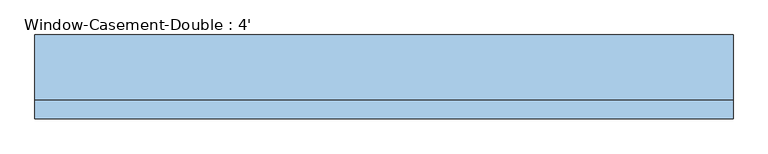
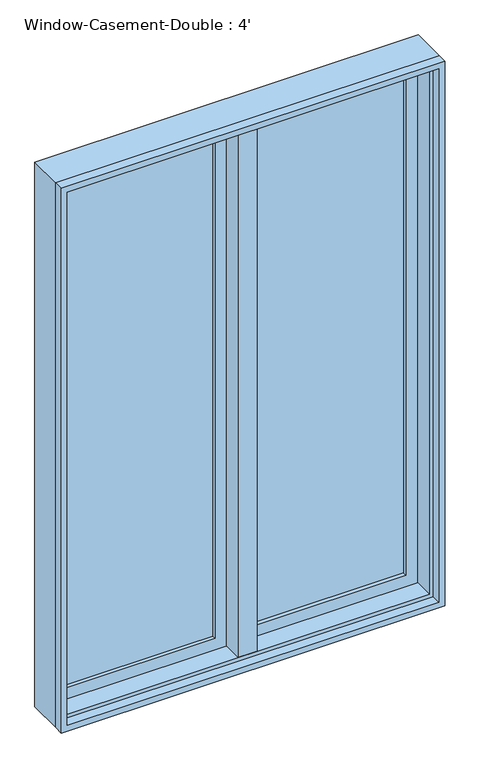
"""IFC4 building model written with IfcOpenShell, lengths in millimetres: window geometry, Window-Casement-Double : 4'."""

from ifc_helpers import new_model, si_unit, frame, origin, place, context, project, spatial, polyline, outline, extrude, faceted_brep, source, transform, mapped, element, save


def window_casement_double_4_52a76413(model_context):
    return source(origin(), model_context, "Body", "SolidModel", [
        faceted_brep([(9.525, 82.55, 2730.5), (-9.525, 82.55, 2730.5), (-9.525, 31.75, 2730.5), (9.525, 31.75, 2730.5), (9.525, 82.55, 927.1), (9.525, 31.75, 927.1), (-9.525, 31.75, 927.1), (-9.525, 82.55, 927.1), (-9.525, 31.75, 946.15), (-9.525, 31.75, 2711.45), (-30.1625, 31.75, 946.15), (-30.1625, 31.75, 2711.45), (-30.1625, -31.75, 946.15), (-30.1625, -31.75, 2711.45), (30.1625, -31.75, 946.15), (30.1625, -31.75, 2711.45), (30.1625, 31.75, 946.15), (30.1625, 31.75, 2711.45), (9.525, 31.75, 946.15), (9.525, 31.75, 2711.45)], [[[0, 1, 2, 3]], [[4, 5, 6, 7]], [[1, 0, 4, 7]], [[2, 1, 7, 6, 8, 9]], [[9, 8, 10, 11]], [[11, 10, 12, 13]], [[13, 12, 14, 15]], [[15, 14, 16, 17]], [[17, 16, 18, 19]], [[0, 3, 19, 18, 5, 4]], [[18, 8, 6, 5]], [[9, 19, 3, 2]], [[8, 18, 16, 14, 12, 10]], [[19, 9, 11, 13, 15, 17]]]),
        extrude(outline(polyline([(-66.675, 63.5), (-66.675, 57.15), (-539.75, 57.15), (-539.75, 63.5), (-66.675, 63.5)])), frame((0.0, 0.0, 984.25), z_axis=(0.0, 0.0, 1.0), x_axis=(1.0, 0.0, 0.0)), (0.0, 0.0, 1.0), 1689.1),
        extrude(outline(polyline([(-539.75, 44.45), (-539.75, 50.8), (-66.675, 50.8), (-66.675, 44.45), (-539.75, 44.45)])), frame((0.0, 0.0, 984.25), z_axis=(0.0, 0.0, 1.0), x_axis=(1.0, 0.0, 0.0)), (0.0, 0.0, 1.0), 1689.1),
        extrude(outline(polyline([(539.75, 63.5), (539.75, 57.15), (66.675, 57.15), (66.675, 63.5), (539.75, 63.5)])), frame((0.0, 0.0, 984.25), z_axis=(0.0, 0.0, 1.0), x_axis=(1.0, 0.0, 0.0)), (0.0, 0.0, 1.0), 1689.1),
        extrude(outline(polyline([(66.675, 44.45), (66.675, 50.8), (539.75, 50.8), (539.75, 44.45), (66.675, 44.45)])), frame((0.0, 0.0, 984.25), z_axis=(0.0, 0.0, 1.0), x_axis=(1.0, 0.0, 0.0)), (0.0, 0.0, 1.0), 1689.1),
        extrude(outline(polyline([(2730.5, -596.9), (927.1, -596.9), (927.1, -9.525), (2730.5, -9.525), (2730.5, -596.9)]), holes=[polyline([(2673.35, -66.675), (984.25, -66.675), (984.25, -539.75), (2673.35, -539.75), (2673.35, -66.675)])]), frame((0.0, 31.75, 0.0), z_axis=(0.0, 1.0, 0.0), x_axis=(0.0, 0.0, 1.0)), (0.0, 0.0, 1.0), 44.45),
        extrude(outline(polyline([(927.1, 596.9), (2730.5, 596.9), (2730.5, 9.525), (927.1, 9.525), (927.1, 596.9)]), holes=[polyline([(984.25, 66.675), (2673.35, 66.675), (2673.35, 539.75), (984.25, 539.75), (984.25, 66.675)])]), frame((0.0, 31.75, 0.0), z_axis=(0.0, 1.0, 0.0), x_axis=(0.0, 0.0, 1.0)), (0.0, 0.0, 1.0), 44.45),
        extrude(outline(polyline([(2743.2, -609.6), (914.4, -609.6), (914.4, 609.6), (2743.2, 609.6), (2743.2, -609.6)]), holes=[polyline([(2724.15, 590.55), (933.45, 590.55), (933.45, -590.55), (2724.15, -590.55), (2724.15, 590.55)])]), frame((0.0, -63.5, 0.0), z_axis=(0.0, 1.0, 0.0), x_axis=(0.0, 0.0, 1.0)), (0.0, 0.0, 1.0), 31.75),
        faceted_brep([(577.85, 31.75, 2711.45), (577.85, -31.75, 2711.45), (-577.85, -31.75, 2711.45), (-577.85, 31.75, 2711.45), (596.9, 82.55, 2730.5), (596.9, 31.75, 2730.5), (-596.9, 31.75, 2730.5), (-596.9, 82.55, 2730.5), (609.6, -31.75, 2743.2), (609.6, 82.55, 2743.2), (-609.6, 82.55, 2743.2), (-609.6, -31.75, 2743.2), (-577.85, -31.75, 946.15), (-577.85, 31.75, 946.15), (-596.9, 31.75, 927.1), (-596.9, 82.55, 927.1), (-609.6, 82.55, 914.4), (-609.6, -31.75, 914.4), (577.85, -31.75, 946.15), (577.85, 31.75, 946.15), (596.9, 31.75, 927.1), (596.9, 82.55, 927.1), (609.6, 82.55, 914.4), (609.6, -31.75, 914.4)], [[[0, 1, 2, 3]], [[4, 5, 6, 7]], [[8, 9, 10, 11]], [[3, 2, 12, 13]], [[7, 6, 14, 15]], [[11, 10, 16, 17]], [[13, 12, 18, 19]], [[15, 14, 20, 21]], [[17, 16, 22, 23]], [[11, 17, 23, 8], [1, 18, 12, 2]], [[19, 18, 1, 0]], [[5, 20, 14, 6], [3, 13, 19, 0]], [[21, 20, 5, 4]], [[23, 22, 9, 8]], [[9, 22, 16, 10], [7, 15, 21, 4]]]),
    ])


if __name__ == "__main__":
    model = new_model("IFC4")
    model_context = context("Model", 3, world=origin())
    ifc_project = project(units=[si_unit("LENGTHUNIT", "METRE", prefix="MILLI")], contexts=[model_context])
    site = spatial("IfcSite", under=ifc_project)
    building = spatial("IfcBuilding", under=site)
    placement = place(None, origin())
    window_casement_double_4_shape = window_casement_double_4_52a76413(model_context)
    element("IfcWindow", 1, ObjectType="Window-Casement-Double : 4'", at=placement, inside=building, context=model_context, shape_type="MappedRepresentation", body=[
        mapped(window_casement_double_4_shape, transform((0.0, 0.0, 0.0), x_axis=(1.0, 0.0, 0.0), y_axis=(0.0, 1.0, 0.0), z_axis=(0.0, 0.0, 1.0))),
    ])
    save(model, "model.ifc")

# Revit data of these elements
# Type "Window-Casement-Double : 4'"
#   Type Mark = "28"
#   Fire Rating = "0.5h"
#   Assembly Code = "B2020100"
#   Analytic Construction = "Double glazing - domestic"
#   Frame Extension [instance default] = 0' - 0 1/4"
#   Window Inset [instance default] = 0' - 0"
#   Wall Thickness [instance default] = 0' - 6"
#   Interior Wall Closure [instance default] = 0' - 2 1/4"
#   Half Width = 2' - 0"
#   Visual Light Transmittance = 0.81
#   Thermal Resistance (R) = 1.8146 (h·ft²·°F)/BTU
#   Solar Heat Gain Coefficient = 0.76
#   Rough Width = 4' - 0 1/2"
#   Rough Height = 6' - 0 1/2"
#   Height = 6' - 0"
#   Heat Transfer Coefficient (U) = 0.5511 BTU/(h·ft²·°F)
#   Exterior Wall Closure [instance default] = 0' - 1 1/4"
#   Extension Jamb [instance default] = 0' - 2 1/4"
#   Default Sill Height = 3' - 0"
#   Width = 4' - 0"
#   Muntin Visibility = yes
#   Interior Trim Visibility [instance default] = yes
#   Exterior Trim Visibility [instance default] = yes
#   Extension Jamb Visibility [instance default] = yes
#   Interior Trim Material = Wood - Stained
#   Muntin Pattern = Muntin Pattern_2x2 : Muntin Pattern_2x2
#   Interior Trim = Trim-Window-Interior-Flat : Picture Frame
#   Interior Frame Material = Wood - Stained
#   Glass Panel Material = Glass
#   Exterior Trim Material = Clad - White
#   Exterior Trim = Trim-Window-Exterior-Flat : with Sill
#   Exterior Frame Material = Clad - White
#   Wall Closure = (empty or 0)
# Element 1 (IfcWindow, "Window-Casement-Double : 4'")
#   Wall Thickness = 0' - 5"
#   Extension Jamb = 0' - 1 1/4"
#   Materials on its faces: "Wood - Stained", "Glass", "Clad - White"
# Materials
#   "Wood - Stained": class "Wood", colour RGB 224 178 126, transparency 0, Cost = 0
#   "Glass": class "Glass", colour RGB 0 128 192, transparency 0.75, Description = "Soda Lime Glass", Cost = 0
#   "Clad - White": class "Wood", colour RGB 242 242 238, transparency 0, Cost = 0
